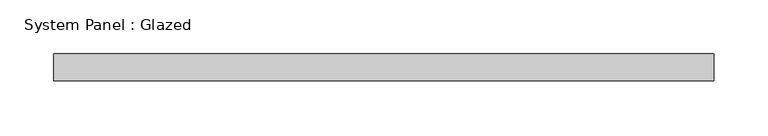
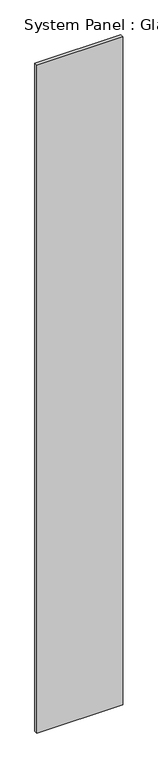
"""IFC4 building model written with IfcOpenShell, lengths in millimetres: plate geometry, System Panel : Glazed."""

from ifc_helpers import new_model, si_unit, origin, origin_with_axes, place, context, project, spatial, polyline, outline, extrude, source, transform, mapped, element, save


def system_panel_glazed_8a9bbf22(model_context):
    return source(origin(), model_context, "Body", "SweptSolid", [
        extrude(outline(polyline([(307.6922868, 19.05), (-307.6922868, 19.05), (-307.6922868, 44.45), (307.6922868, 44.45), (307.6922868, 19.05)])), origin_with_axes(), (0.0, 0.0, 1.0), 5054.6),
    ])


if __name__ == "__main__":
    model = new_model("IFC4")
    model_context = context("Model", 3, world=origin())
    ifc_project = project(units=[si_unit("LENGTHUNIT", "METRE", prefix="MILLI")], contexts=[model_context])
    site = spatial("IfcSite", under=ifc_project)
    building = spatial("IfcBuilding", under=site)
    placement = place(None, origin())
    system_panel_glazed_shape = system_panel_glazed_8a9bbf22(model_context)
    element("IfcPlate", 1, ObjectType="System Panel : Glazed", at=placement, inside=building, context=model_context, shape_type="MappedRepresentation", body=[
        mapped(system_panel_glazed_shape, transform((0.0, 0.0, 0.0), x_axis=(1.0, 0.0, 0.0), y_axis=(0.0, 1.0, 0.0), z_axis=(0.0, 0.0, 1.0))),
    ])
    save(model, "model.ifc")

# Revit data of these elements
# Type "System Panel : Glazed"
#   Construction Type Id = "GSP4R"
#   Analytic Construction = "1/8 in Pilkington single glazing"
#   Visual Light Transmittance = 0.9
#   Solar Heat Gain Coefficient = 0.86
#   Heat Transfer Coefficient (U) = 1.18115 BTU/(h·ft²·°F)
# Element 1 (IfcPlate, "System Panel : Glazed")
#   Materials on its faces: "Glass"
# Materials
#   "Glass": class "Glass", colour RGB 0 128 192, transparency 0.75, Description = "Soda Lime Glass", Cost = 0
